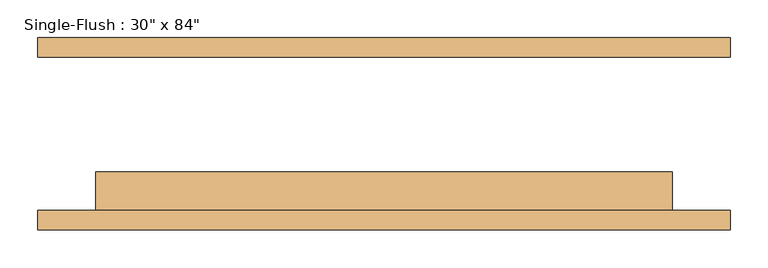
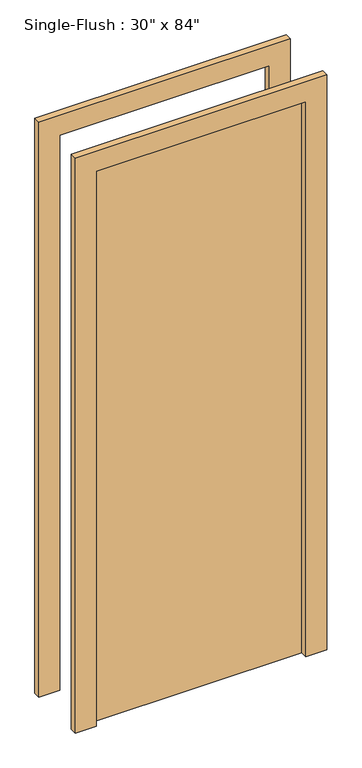
"""IFC4 building model written with IfcOpenShell, lengths in millimetres: door geometry."""

from ifc_helpers import new_model, si_unit, frame, origin, origin_with_axes, place, context, project, spatial, polyline, outline, extrude, source, transform, mapped, element, save


def door_4314e8ec(model_context):
    return source(origin(), model_context, "Body", "SweptSolid", [
        extrude(outline(polyline([(2209.8, -457.2), (0.0, -457.2), (0.0, -381.0), (2133.6, -381.0), (2133.6, 381.0), (0.0, 381.0), (0.0, 457.2), (2209.8, 457.2), (2209.8, -457.2)])), frame((0.0, -127.0, 0.0), z_axis=(0.0, 1.0, 0.0), x_axis=(0.0, 0.0, 1.0)), (0.0, 0.0, 1.0), 25.4),
        extrude(outline(polyline([(2209.8, 457.2), (2209.8, -457.2), (0.0, -457.2), (0.0, -381.0), (2133.6, -381.0), (2133.6, 381.0), (0.0, 381.0), (0.0, 457.2), (2209.8, 457.2)])), frame((0.0, 101.6, 0.0), z_axis=(0.0, 1.0, 0.0), x_axis=(0.0, 0.0, 1.0)), (0.0, 0.0, 1.0), 25.4),
        extrude(outline(polyline([(381.0, -50.8), (381.0, -101.6), (-381.0, -101.6), (-381.0, -50.8), (381.0, -50.8)])), origin_with_axes(), (0.0, 0.0, 1.0), 2133.6),
    ])


if __name__ == "__main__":
    model = new_model("IFC4")
    model_context = context("Model", 3, world=origin())
    ifc_project = project(units=[si_unit("LENGTHUNIT", "METRE", prefix="MILLI")], contexts=[model_context])
    site = spatial("IfcSite", under=ifc_project)
    building = spatial("IfcBuilding", under=site)
    placement = place(None, origin())
    door_shape = door_4314e8ec(model_context)
    element("IfcDoor", 1, ObjectType="Single-Flush : 30\" x 84\"", at=placement, inside=building, context=model_context, shape_type="MappedRepresentation", body=[
        mapped(door_shape, transform((0.0, 0.0, 0.0), x_axis=(1.0, 0.0, 0.0), y_axis=(0.0, 1.0, 0.0), z_axis=(0.0, 0.0, 1.0))),
    ])
    save(model, "model.ifc")

# Revit data of these elements
# Type "Single-Flush : 30\" x 84\""
#   Type Mark = "4"
#   Construction Type Id = "MDOOR"
#   Assembly Code = "C1020"
#   Analytic Construction = "Metal"
#   Thickness = 0' - 2"
#   Heat Transfer Coefficient (U) = 0.651978 BTU/(h·ft²·°F)
#   Height = 7' - 0"
#   Trim Projection Ext = 0' - 1"
#   Trim Projection Int = 0' - 1"
#   Trim Width = 0' - 3"
#   Width = 2' - 6"
#   Define Thermal Properties by = 1
#   Door Material = Door - Panel
#   Frame Material = Door - Frame
#   Visual Light Transmittance = 0
#   Solar Heat Gain Coefficient = 0
#   Function = (empty or 0)
#   Wall Closure = (empty or 0)
# Element 1 (IfcDoor, "Single-Flush : 30\" x 84\"")
#   Materials on its faces: "Door - Frame", "Door - Panel"
# Materials
#   "Door - Panel": class "Wood", colour RGB 210 159 95, transparency 0
#   "Door - Frame": colour RGB 118 70 51, transparency 0
